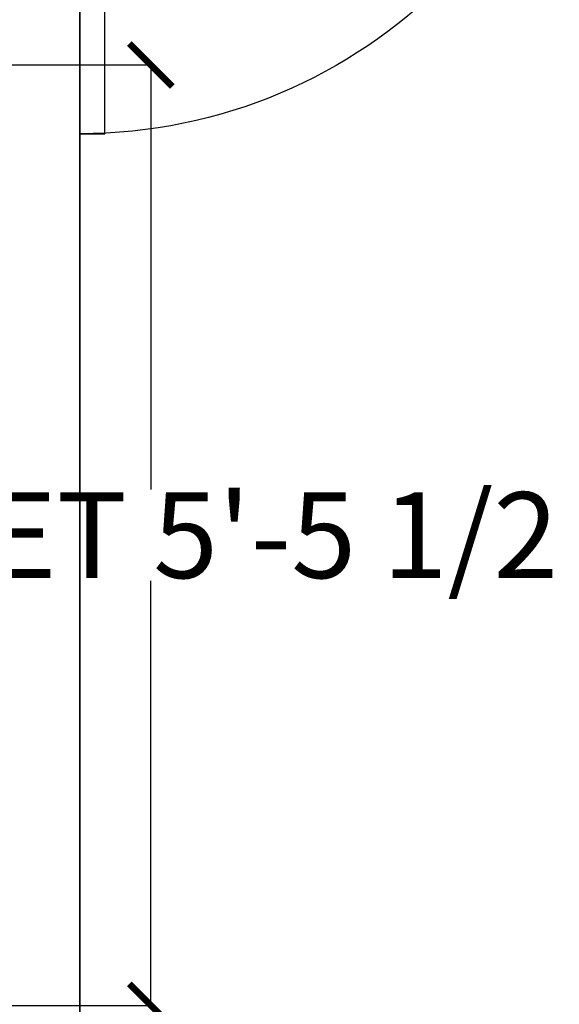
# Model space of a CAD drawing. Units: inches. Extents: x 844 to 2234, y 346 to 1084.
# Tile 89 of 93: x 2031 to 2069, y 669 to 737. Entities that reach past the tile are written whole.
import ezdxf

# ---------------------------------------------------------------- set-up
doc = ezdxf.new("R2010")
doc.units = ezdxf.units.IN
doc.header["$MEASUREMENT"] = 0
for name, color, linetype, lineweight in [('A-ANNO-DIMS', 2, 'Continuous', 18), ('A-WALL', 7, 'Continuous', 35), ('doors', 170, 'Continuous', 25)]:
    doc.layers.add(name, color=color, linetype=linetype, lineweight=lineweight)
doc.styles.get("Standard").update_dxf_attribs({"font": 'arial.ttf'})
doc.dimstyles.get("Standard").update_dxf_attribs({"dimtxt": 6, "dimasz": 3, "dimexe": 0.18, "dimexo": 0.0625, "dimgap": 0.09, "dimtad": 0, "dimtih": 1, "dimtoh": 1, "dimdec": 1, "dimzin": 0, "dimdsep": 46, "dimlunit": 3, "dimtxsty": 'Standard', "dimblk": 'ARCHTICK', "dimcen": 0.09, "dimadec": 0, "dimazin": 0, "dimtfac": 1, "dimtdec": 1, "dimtofl": 0, "dimtmove": 0, "dimatfit": 3, "dimfxl": 1, "dimtolj": 1, "dimtzin": 0, "dimarcsym": 0})

# ---------------------------------------------------------------- blocks, each defined once
blk = doc.blocks.new('*U2')
for p, q in [((0, 0), (0, -6)), ((36, 0), (36, -6))]:
    blk.add_line(p, q)
blk.add_lwpolyline([(0, 0), (0, 36), (1.75, 36), (1.75, 0)], close=True)
blk.add_arc((0, 0), 36, 0, 90)
blk = doc.blocks.new('_ArchTick')
at = {"color": 0, "linetype": 'ByBlock', "const_width": 0.15}
blk.add_lwpolyline([(-0.5, -0.5), (0.5, 0.5)], dxfattribs=at)
blk = doc.blocks.new('*D121')
at = {"layer": 'A-ANNO-DIMS', "color": 0, "lineweight": -2, "transparency": 16777216}
for p, q in [((2030.272, 734.263), (2040.245, 734.263)), ((2040.065, 734.263), (2040.065, 704.604)), ((2040.065, 668.557), (2040.065, 698.216)), ((2030.272, 668.557), (2040.245, 668.557))]:
    blk.add_line(p, q, dxfattribs=at)
at = {"layer": 'Defpoints', "color": 0, "transparency": 16777216}
for p in [(2030.209, 734.263), (2040.065, 734.263), (2030.209, 668.557)]:
    blk.add_point(p, dxfattribs=at)
at = {"layer": 'A-ANNO-DIMS', "color": 0, "lineweight": -2, "transparency": 16777216, "xscale": 3, "yscale": 3, "zscale": 3}
for p, rotation in [((2040.065, 734.263), 90), ((2040.065, 668.557), 270)]:
    blk.add_blockref('_ArchTick', p, dxfattribs=dict(at, rotation=rotation))
at = {"layer": 'A-ANNO-DIMS', "color": 0, "transparency": 16777216, "insert": (2040.065, 701.41), "char_height": 6, "attachment_point": 5}
blk.add_mtext('\\A1;LOUNGE SET 5\'-5 1/2" TYP.', dxfattribs=at)

msp = doc.modelspace()

# ---------------------------------------------------------------- linework, layer by layer
at = {"layer": 'A-WALL'}
msp.add_line((2035.099, 766.455), (2035.099, 634.455), dxfattribs=at)

# ---------------------------------------------------------------- block references
at = {"layer": 'doors', "xscale": -1, "rotation": 180}
msp.add_blockref('*U2', (2035.099, 765.455), dxfattribs=at)

# ---------------------------------------------------------------- dimensions: what is measured, and where the dimension line sits
at = {"layer": 'A-ANNO-DIMS'}
dim = msp.add_linear_dim(base=(2040.065, 734.263), p1=(2030.209, 668.557), p2=(2030.209, 734.263), angle=90, text='LOUNGE SET <> TYP.', dimstyle='Standard', override={"dimdec": 1, "dimlfac": 1, "dimrnd": 0, "dimzin": 1, "dimdsep": 46, "dimlunit": 4, "dimfrac": 2}, dxfattribs=at)
dim.commit()
dim.dimension.update_dxf_attribs({"geometry": '*D121', "text_midpoint": (2040.065, 701.41)})

doc.saveas('drawing.dxf')
